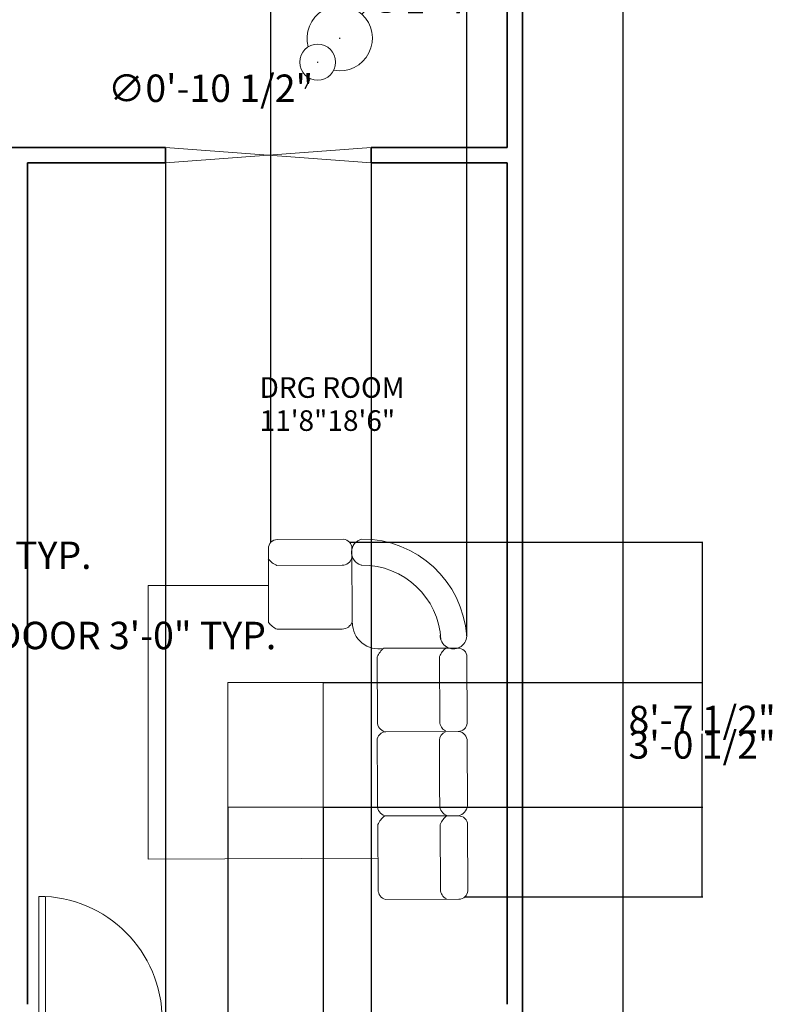
# Model space of a CAD drawing. Units: inches. Extents: x -438 to 102, y -60 to 1091.
# Tile 3 of 20: x -118 to 102, y 205 to 492. Entities that reach past the tile are written whole.
import ezdxf

# ---------------------------------------------------------------- set-up
doc = ezdxf.new("R2010")
doc.units = ezdxf.units.IN
doc.header["$MEASUREMENT"] = 0
for name, color, linetype, lineweight, true_color in [('A-ANNO-DIMS', 217, 'Continuous', 18, 0x93278f), ('A-DOOR', 30, 'Continuous', 18, 0xf26722), ('A-WALL', 2, 'Continuous', 35, 0xf1eb1f), ('C-PROP', 2, 'Continuous', 35, 0xf1eb1f)]:
    doc.layers.add(name, color=color, linetype=linetype, lineweight=lineweight, true_color=true_color)
for name, color, linetype, lineweight in [('A-AREA-IDEN', 4, 'Continuous', 18), ('A-GLAZ', 4, 'Continuous', 18), ('Furniture', 7, 'Continuous', 15)]:
    doc.layers.add(name, color=color, linetype=linetype, lineweight=lineweight)
doc.styles.get("Standard").update_dxf_attribs({"font": 'arial.ttf'})
doc.dimstyles.get("Standard").update_dxf_attribs({"dimtxt": 8, "dimasz": 0.18, "dimexe": 0.18, "dimexo": 0.0625, "dimgap": 0.09, "dimtad": 0, "dimtih": 1, "dimtoh": 1, "dimdec": 4, "dimzin": 0, "dimdsep": 46, "dimlunit": 3, "dimtxsty": 'Standard', "dimcen": 0.09, "dimadec": 0, "dimazin": 0, "dimtfac": 1, "dimtdec": 4, "dimtofl": 0, "dimtmove": 0, "dimatfit": 3, "dimfxl": 1, "dimtolj": 1, "dimtzin": 0, "dimarcsym": 0})

# ---------------------------------------------------------------- blocks, each defined once
blk = doc.blocks.new('*D5')
at = {"layer": 'A-ANNO-DIMS', "color": 0, "lineweight": -2, "transparency": 16777216}
for p, q in [((28.92, 1027), (58.42, 1027)), ((58.24, 1026.82), (58.24, 519.68)), ((58.24, 4.18), (58.24, 511.32)), ((28.92, 4), (58.42, 4))]:
    blk.add_line(p, q, dxfattribs=at)
at = {"layer": 'A-ANNO-DIMS', "color": 0, "transparency": 16777216}
for points in [[(58.21, 1026.82), (58.27, 1026.82), (58.24, 1027)], [(58.21, 4.18), (58.27, 4.18), (58.24, 4)]]:
    blk.add_solid(points, dxfattribs=at)
at = {"layer": 'Defpoints', "color": 0, "transparency": 16777216}
for p in [(28.85, 1027), (28.85, 4), (58.24, 4)]:
    blk.add_point(p, dxfattribs=at)
at = {"layer": 'A-ANNO-DIMS', "color": 0, "transparency": 16777216, "insert": (58.24, 515.5), "char_height": 8, "attachment_point": 5}
blk.add_mtext('\\A1;85\'-3.0000"', dxfattribs=at)
blk = doc.blocks.new('DOOR-SWING-36')
for p, q in [((-36, 0), (0, 0)), ((-2, 0), (-2, -36)), ((0, 0), (0, -36))]:
    blk.add_line(p, q)
blk.add_arc((0, 0), 36, 180, 270)
blk = doc.blocks.new('*D20')
at = {"layer": 'A-ANNO-DIMS', "color": 0, "lineweight": -2, "transparency": 16777216}
for p, q in [((-162.74, 317.94), (-162.74, 312.42)), ((-126.74, 317.94), (-126.74, 312.42)), ((-162.56, 312.6), (-126.92, 312.6)), ((-126.74, 312.6), (-126.56, 312.6))]:
    blk.add_line(p, q, dxfattribs=at)
at = {"layer": 'A-ANNO-DIMS', "color": 0, "transparency": 16777216}
for points in [[(-162.56, 312.63), (-162.56, 312.57), (-162.74, 312.6)], [(-126.92, 312.63), (-126.92, 312.57), (-126.74, 312.6)]]:
    blk.add_solid(points, dxfattribs=at)
at = {"layer": 'Defpoints', "color": 0, "transparency": 16777216}
for p in [(-162.74, 318), (-126.74, 318), (-126.74, 312.6)]:
    blk.add_point(p, dxfattribs=at)
at = {"layer": 'A-ANNO-DIMS', "color": 0, "transparency": 16777216, "insert": (-83.97, 312.6), "char_height": 8, "attachment_point": 5}
blk.add_mtext('\\A1;DOOR 3\'-0" TYP.', dxfattribs=at)
blk = doc.blocks.new('*D21')
at = {"layer": 'A-ANNO-DIMS', "color": 0, "lineweight": -2, "transparency": 16777216}
for p, q in [((-126.67, 354), (-121.16, 354)), ((-121.34, 353.82), (-121.34, 340.18)), ((-121.34, 318.18), (-121.34, 331.82)), ((-126.67, 318), (-121.16, 318))]:
    blk.add_line(p, q, dxfattribs=at)
at = {"layer": 'A-ANNO-DIMS', "color": 0, "transparency": 16777216}
for points in [[(-121.37, 353.82), (-121.31, 353.82), (-121.34, 354)], [(-121.37, 318.18), (-121.31, 318.18), (-121.34, 318)]]:
    blk.add_solid(points, dxfattribs=at)
at = {"layer": 'Defpoints', "color": 0, "transparency": 16777216}
for p in [(-126.74, 354), (-121.34, 354), (-126.74, 318)]:
    blk.add_point(p, dxfattribs=at)
at = {"layer": 'A-ANNO-DIMS', "color": 0, "transparency": 16777216, "insert": (-121.34, 336), "char_height": 8, "attachment_point": 5}
blk.add_mtext('\\A1;3\'-0" TYP.', dxfattribs=at)
blk = doc.blocks.new('*D31')
at = {"layer": 'A-ANNO-DIMS', "color": 0, "lineweight": -2, "transparency": 16777216}
for p, q in [((-75.33, 454.94), (-75.33, -48.58)), ((-15.33, 454.94), (-15.33, -48.58)), ((-75.15, -48.4), (-56.05, -48.4)), ((-15.51, -48.4), (-34.6, -48.4))]:
    blk.add_line(p, q, dxfattribs=at)
at = {"layer": 'A-ANNO-DIMS', "color": 0, "transparency": 16777216}
for points in [[(-75.15, -48.37), (-75.15, -48.43), (-75.33, -48.4)], [(-15.51, -48.37), (-15.51, -48.43), (-15.33, -48.4)]]:
    blk.add_solid(points, dxfattribs=at)
at = {"layer": 'Defpoints', "color": 0, "transparency": 16777216}
for p in [(-75.33, 455), (-15.33, 455), (-15.33, -48.4)]:
    blk.add_point(p, dxfattribs=at)
at = {"layer": 'A-ANNO-DIMS', "color": 0, "transparency": 16777216, "insert": (-45.33, -48.4), "char_height": 8, "attachment_point": 5}
blk.add_mtext('\\A1;5\'-0"', dxfattribs=at)
blk = doc.blocks.new('*D35')
at = {"layer": 'A-ANNO-DIMS', "color": 0, "lineweight": -2, "transparency": 16777216}
for p, q in [((-57.12, 262.42), (-57.12, -48.58)), ((-29.37, 262.42), (-29.37, -48.58)), ((-56.94, -48.4), (-54.03, -48.4)), ((-29.55, -48.4), (-32.45, -48.4))]:
    blk.add_line(p, q, dxfattribs=at)
at = {"layer": 'A-ANNO-DIMS', "color": 0, "transparency": 16777216}
for points in [[(-56.94, -48.37), (-56.94, -48.43), (-57.12, -48.4)], [(-29.55, -48.37), (-29.55, -48.43), (-29.37, -48.4)]]:
    blk.add_solid(points, dxfattribs=at)
at = {"layer": 'Defpoints', "color": 0, "transparency": 16777216}
for p in [(-57.12, 262.49), (-29.37, 262.49), (-29.37, -48.4)]:
    blk.add_point(p, dxfattribs=at)
at = {"layer": 'A-ANNO-DIMS', "color": 0, "transparency": 16777216, "insert": (-43.24, -48.4), "char_height": 8, "attachment_point": 5}
blk.add_mtext('\\A1;2\'-4"', dxfattribs=at)
blk = doc.blocks.new('*D36')
at = {"layer": 'A-ANNO-DIMS', "color": 0, "lineweight": -2, "transparency": 16777216}
for p, q in [((-29.3, 298.85), (81.43, 298.85)), ((81.25, 298.67), (81.25, 284.9)), ((81.25, 262.67), (81.25, 276.44)), ((-29.3, 262.49), (81.43, 262.49))]:
    blk.add_line(p, q, dxfattribs=at)
at = {"layer": 'A-ANNO-DIMS', "color": 0, "transparency": 16777216}
for points in [[(81.22, 298.67), (81.28, 298.67), (81.25, 298.85)], [(81.22, 262.67), (81.28, 262.67), (81.25, 262.49)]]:
    blk.add_solid(points, dxfattribs=at)
at = {"layer": 'Defpoints', "color": 0, "transparency": 16777216}
for p in [(-29.37, 298.85), (81.25, 298.85), (-29.37, 262.49)]:
    blk.add_point(p, dxfattribs=at)
at = {"layer": 'A-ANNO-DIMS', "color": 0, "transparency": 16777216, "insert": (81.25, 280.67), "char_height": 8, "attachment_point": 5}
blk.add_mtext('\\A1;3\'-0 1/2"', dxfattribs=at)
blk = doc.blocks.new('*D49')
at = {"layer": 'A-ANNO-DIMS', "color": 0, "lineweight": -2, "transparency": 16777216}
for p, q in [((-44.57, 339.86), (-44.57, 1079.58)), ((-44.39, 1079.4), (-26.89, 1079.4)), ((12.37, 1079.4), (-5.13, 1079.4)), ((12.55, 312.51), (12.55, 1079.58))]:
    blk.add_line(p, q, dxfattribs=at)
at = {"layer": 'A-ANNO-DIMS', "color": 0, "transparency": 16777216}
for points in [[(-44.39, 1079.43), (-44.39, 1079.37), (-44.57, 1079.4)], [(12.37, 1079.43), (12.37, 1079.37), (12.55, 1079.4)]]:
    blk.add_solid(points, dxfattribs=at)
at = {"layer": 'Defpoints', "color": 0, "transparency": 16777216}
for p in [(12.55, 1079.4), (-44.57, 339.79), (12.55, 312.44)]:
    blk.add_point(p, dxfattribs=at)
at = {"layer": 'A-ANNO-DIMS', "color": 0, "transparency": 16777216, "insert": (-16.01, 1079.4), "char_height": 8, "attachment_point": 5}
blk.add_mtext('\\A1;4\'-9"', dxfattribs=at)
blk = doc.blocks.new('*D50')
at = {"layer": 'A-ANNO-DIMS', "color": 0, "lineweight": -2, "transparency": 16777216}
for p, q in [((-21.61, 339.82), (81.43, 339.82)), ((81.25, 339.64), (81.25, 292.31)), ((81.25, 236.53), (81.25, 283.86)), ((12.11, 236.35), (81.43, 236.35))]:
    blk.add_line(p, q, dxfattribs=at)
at = {"layer": 'A-ANNO-DIMS', "color": 0, "transparency": 16777216}
for points in [[(81.22, 339.64), (81.28, 339.64), (81.25, 339.82)], [(81.22, 236.53), (81.28, 236.53), (81.25, 236.35)]]:
    blk.add_solid(points, dxfattribs=at)
at = {"layer": 'Defpoints', "color": 0, "transparency": 16777216}
for p in [(-21.67, 339.82), (12.05, 236.35), (81.25, 236.35)]:
    blk.add_point(p, dxfattribs=at)
at = {"layer": 'A-ANNO-DIMS', "color": 0, "transparency": 16777216, "insert": (81.25, 288.09), "char_height": 8, "attachment_point": 5}
blk.add_mtext('\\A1;8\'-7 1/2"', dxfattribs=at)
blk = doc.blocks.new('*D62')
at = {"layer": 'A-ANNO-DIMS', "color": 0, "lineweight": -2, "transparency": 16777216}
for p, q in [((-14.2, 498.06), (-17.94, 493.99)), ((-14.02, 498.06), (-14.2, 498.06)), ((-24.59, 486.85), (-24.41, 486.85)), ((-24.5, 486.76), (-24.5, 486.94))]:
    blk.add_line(p, q, dxfattribs=at)
at = {"layer": 'A-ANNO-DIMS', "color": 0, "transparency": 16777216}
blk.add_solid([(-17.96, 494.01), (-17.92, 493.97), (-18.06, 493.86)], dxfattribs=at)
at = {"layer": 'Defpoints', "color": 0, "transparency": 16777216}
for p in [(-18.06, 493.86), (-30.94, 479.85)]:
    blk.add_point(p, dxfattribs=at)
at = {"layer": 'A-ANNO-DIMS', "color": 0, "transparency": 16777216, "insert": (1.06, 498.06), "char_height": 8, "attachment_point": 5}
blk.add_mtext('\\A1;∅1\'-7"', dxfattribs=at)
blk = doc.blocks.new('*D63')
at = {"layer": 'A-ANNO-DIMS', "color": 0, "lineweight": -2, "transparency": 16777216}
for p, q in [((-31.03, 479.85), (-30.85, 479.85)), ((-30.94, 479.76), (-30.94, 479.94)), ((-34.5, 472.25), (-33.24, 474.94)), ((-34.68, 472.25), (-34.5, 472.25))]:
    blk.add_line(p, q, dxfattribs=at)
at = {"layer": 'A-ANNO-DIMS', "color": 0, "transparency": 16777216}
blk.add_solid([(-33.27, 474.95), (-33.21, 474.92), (-33.17, 475.1)], dxfattribs=at)
at = {"layer": 'Defpoints', "color": 0, "transparency": 16777216}
for p in [(-28.72, 484.6), (-33.17, 475.1)]:
    blk.add_point(p, dxfattribs=at)
at = {"layer": 'A-ANNO-DIMS', "color": 0, "transparency": 16777216, "insert": (-62.18, 472.25), "char_height": 8, "attachment_point": 5}
blk.add_mtext('\\A1;∅0\'-10 1/2"', dxfattribs=at)

msp = doc.modelspace()

# ---------------------------------------------------------------- linework, layer by layer
at = {"layer": 'A-GLAZ'}
for p, q in [((-75.32797, 454.99939), (-15.32797, 450.49939)), ((-15.32797, 454.99939), (-75.32797, 450.49939))]:
    msp.add_line(p, q, dxfattribs=at)
at = {"layer": 'A-WALL'}
for p, q in [((24.35351, 454.99939), (24.35351, 660.99939)), ((-75.32797, 454.99939), (-120.14649, 454.99939)), ((-75.32797, 454.99939), (-75.32797, 450.49939)), ((24.35351, 454.99939), (-15.32797, 454.99939)), ((-15.32797, 454.99939), (-15.32797, 450.49939)), ((-115.64649, 204.99939), (-115.64649, 450.49939)), ((-75.32797, 450.49939), (-115.64649, 450.49939)), ((24.35351, 450.49939), (-15.32797, 450.49939)), ((24.35351, 204.99939), (24.35351, 450.49939))]:
    msp.add_line(p, q, dxfattribs=at)
at = {"layer": 'C-PROP'}
msp.add_line((28.85351, 3.99939), (28.85351, 1026.99939), dxfattribs=at)
at = {"layer": 'Furniture'}
for p, q in [((-23.4149, 340.67042), (-42.73083, 340.58956)), ((-45.29383, 316.39021), (-45.27294, 337.91595)), ((-20.87185, 316.60341), (-20.9615, 338.01773)), ((-20.94975, 335.21), (-20.95007, 335.28657)), ((-42.81011, 333.0103), (-23.82721, 333.08977)), ((-18.27293, 333.15103), (-18.01344, 333.15212)), ((-45.28338, 327.15308), (-80.4235, 327.15308)), ((-80.4235, 327.15308), (-80.4235, 247.31133)), ((-42.73221, 314.40371), (-23.74931, 314.48318)), ((9.94023, 308.90303), (-11.58551, 308.92392)), ((-13.57201, 306.36231), (-13.49253, 287.37941)), ((4.60596, 306.43841), (4.68544, 287.45551)), ((12.69471, 287.04499), (12.61384, 306.36092)), ((-11.3723, 284.50194), (10.04201, 284.5916)), ((10.2639, 284.59717), (-11.03946, 284.50798)), ((-13.58073, 281.94404), (-13.52125, 267.73462)), ((4.59724, 282.02014), (4.65673, 267.81072)), ((12.79554, 262.96022), (12.717, 281.7211)), ((-13.52125, 267.73462), (-13.50126, 262.96114)), ((4.65673, 267.81072), (4.67671, 263.03724)), ((10.14517, 259.95177), (-11.38057, 259.97267)), ((-13.36707, 257.41105), (-13.28759, 238.42815)), ((4.8109, 257.48715), (4.89038, 238.50425)), ((12.89965, 238.09373), (12.81878, 257.40967)), ((-80.4235, 247.31133), (-13.32596, 247.59224)), ((-11.16736, 235.55069), (10.24695, 235.64034))]:
    msp.add_line(p, q, dxfattribs=at)
msp.add_lwpolyline([(-57.12044, 298.8505), (-29.36624, 298.8505), (-29.36624, 262.4853), (-57.12044, 262.4853)], close=True, dxfattribs=at)
msp.add_circle((-30.94195, 479.84838), 5.24292, dxfattribs=at)
for centre, radius, start, end in [((-24.50081, 486.85219), 9.51534, 259.3798673, 195.4129607), ((-42.72013, 338.03404), 2.55554, 90.239874, 182.6486898), ((-23.63439, 338.00654), 2.67291, 0.239874, 85.2896272), ((-17.15873, 336.9061), 3.91689, 102.665949, 253.4733622), ((-17.91724, 310.1748), 30.55304, 4.2269093, 90.1881535), ((-40.40548, 338.75597), 6.22857, 217.1236759, 247.2901016), ((-23.8399, 336.11967), 3.02993, 270.239874, 342.5286437), ((-17.91724, 310.1748), 22.97752, 3.1558112, 90.239874), ((-40.32758, 320.14938), 6.22857, 217.1236759, 247.2901016), ((-23.762, 317.51308), 3.02993, 270.239874, 342.5286437), ((-13.15912, 316.35529), 7.65685, 180.239874, 280.8404981), ((8.68418, 312.56068), 3.87068, 178.252002, 358.252002), ((-7.82633, 303.95767), 6.22857, 127.1236759, 157.2901016), ((10.35164, 304.03378), 6.22857, 127.1236759, 157.2901016), ((10.05833, 306.35022), 2.55554, 0.239874, 92.6486898), ((-10.46263, 287.39209), 3.02993, 180.239874, 252.5286437), ((7.71534, 287.4682), 3.02993, 180.239874, 244.3141926), ((-11.02877, 281.95601), 2.55199, 90.239874, 180.2688351), ((7.1492, 282.03212), 2.55199, 106.9976124, 180.2688351), ((10.03082, 287.26449), 2.67291, 270.239874, 355.2896272), ((9.7901, 281.70884), 2.92693, 0.239874, 80.6840303), ((-10.31645, 262.97447), 3.18484, 180.239874, 250.4809972), ((7.86152, 263.05058), 3.18484, 180.239874, 250.4809972), ((9.07361, 263.56747), 3.77114, 286.5078661, 350.733565), ((-7.62139, 255.00642), 6.22857, 127.1236759, 157.2901016), ((10.55658, 255.08252), 6.22857, 127.1236759, 157.2901016), ((10.26327, 257.39897), 2.55554, 0.239874, 92.6486898), ((-10.25769, 238.44083), 3.02993, 180.239874, 252.5286437), ((7.92028, 238.51694), 3.02993, 180.239874, 244.3141926), ((10.23576, 238.31323), 2.67291, 270.239874, 355.2896272)]:
    msp.add_arc(centre, radius, start, end, dxfattribs=at)

# ---------------------------------------------------------------- block references
at = {"layer": 'A-DOOR', "rotation": 180}
msp.add_blockref('DOOR-SWING-36', (-112.33294, 200.49939), dxfattribs=at)

# ---------------------------------------------------------------- texts
at = {"layer": 'A-AREA-IDEN'}
for s, p in [('DRG ROOM', (-47.89091, 381.93012)), ('11\'8"18\'6"', (-47.89091, 372.29165))]:
    msp.add_text(s, height=6, dxfattribs=at).set_placement(p)

# ---------------------------------------------------------------- dimensions: what is measured, and where the dimension line sits
at = {"layer": 'A-ANNO-DIMS'}
for base, p1, p2, picture, middle in [((12.55306, 1079.39939), (-44.57214, 339.79496), (12.55306, 312.44261), '*D49', (-16.00954, 1079.39939)), ((-15.32797, -48.40061), (-75.32797, 454.99939), (-15.32797, 454.99939), '*D31', (-45.32797, -48.40061)), ((-29.36624, -48.40061), (-57.12044, 262.4853), (-29.36624, 262.4853), '*D35', (-43.24334, -48.40061))]:
    dim = msp.add_linear_dim(base=base, p1=p1, p2=p2, dimstyle='Standard', override={"dimdec": 1, "dimlfac": 1, "dimrnd": 0, "dimzin": 1, "dimdsep": 46, "dimlunit": 4, "dimfrac": 2}, dxfattribs=at)
    dim.commit()
    dim.dimension.update_dxf_attribs({"geometry": picture, "text_midpoint": middle})
for base, p1, p2, override, picture, middle in [((58.24207, 3.99939), (28.85351, 1026.99939), (28.85351, 3.99939), {"dimclrd": 0, "dimclre": 0, "dimclrt": 0}, '*D5', (58.24207, 515.49939)), ((81.25351, 236.35092), (-21.67208, 339.82142), (12.05064, 236.35092), {"dimdec": 1, "dimlfac": 1, "dimrnd": 0, "dimzin": 1, "dimdsep": 46, "dimlunit": 4, "dimfrac": 2}, '*D50', (81.25351, 288.08617)), ((81.25351, 298.8505), (-29.36624, 262.4853), (-29.36624, 298.8505), {"dimdec": 1, "dimlfac": 1, "dimrnd": 0, "dimzin": 1, "dimdsep": 46, "dimlunit": 4, "dimfrac": 2}, '*D36', (81.25351, 280.6679))]:
    dim = msp.add_linear_dim(base=base, p1=p1, p2=p2, angle=90, dimstyle='Standard', override=override, dxfattribs=at)
    dim.commit()
    dim.dimension.update_dxf_attribs({"geometry": picture, "text_midpoint": middle})
for p1, p2, picture, middle in [((-30.94177, 479.84822), (-18.05985, 493.85616), '*D62', (1.05972, 498.05855)), ((-28.71826, 484.59638), (-33.16564, 475.10039), '*D63', (-62.18323, 472.2516))]:
    dim = msp.add_diameter_dim_2p(p1=p1, p2=p2, dimstyle='Standard', override={"dimdec": 1, "dimlfac": 1, "dimrnd": 0, "dimzin": 1, "dimdsep": 46, "dimlunit": 4, "dimfrac": 2}, dxfattribs=at)
    dim.commit()
    dim.dimension.update_dxf_attribs({"geometry": picture, "text_midpoint": middle, "dimtype": 163})
dim = msp.add_linear_dim(base=(-121.33521, 353.99939), p1=(-126.73521, 317.99939), p2=(-126.73521, 353.99939), angle=90, text='<> TYP.', dimstyle='Standard', override={"dimdec": 1, "dimlfac": 1, "dimrnd": 0, "dimzin": 1, "dimdsep": 46, "dimlunit": 4, "dimfrac": 2}, dxfattribs=at)
dim.commit()
dim.dimension.update_dxf_attribs({"geometry": '*D21', "text_midpoint": (-121.33521, 335.99939)})
dim = msp.add_linear_dim(base=(-126.73521, 312.59939), p1=(-162.73521, 317.99939), p2=(-126.73521, 317.99939), text='DOOR <> TYP.', dimstyle='Standard', override={"dimdec": 1, "dimlfac": 1, "dimrnd": 0, "dimzin": 1, "dimdsep": 46, "dimlunit": 4, "dimfrac": 2}, dxfattribs=at)
dim.commit()
dim.dimension.update_dxf_attribs({"geometry": '*D20', "text_midpoint": (-83.96589, 312.59939)})

doc.saveas('drawing.dxf')
